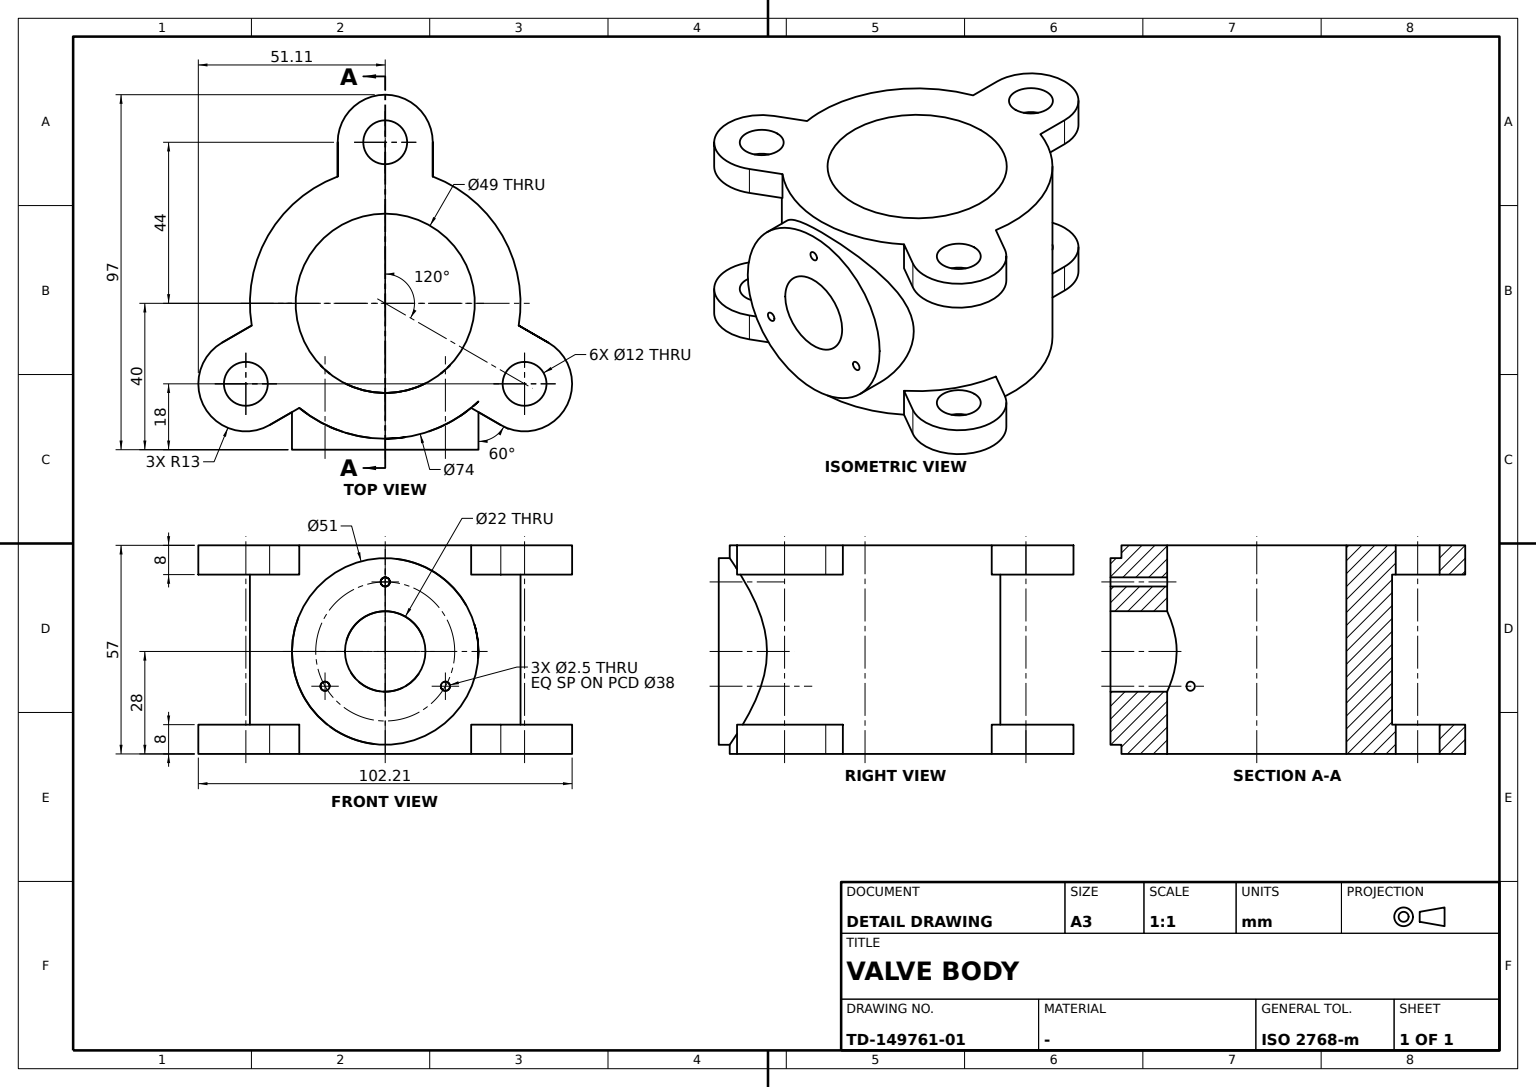
CATIA V5 part; units mm, degrees
ref_plane "Plane1" through (-40, 0, 0) normal (1, 0, 0) x (0, 1, 0)
sketch "Sketch1" plane through (0, 0, 0) normal (0, 0, 1) x (1, 0, 0)
  circle A0 centre (0, 0) radius 37
  dimension "radius A0" = 37
extrude "Pad1" add sketch "Sketch1" along normal blind 57
sketch "Sketch2" plane through (0, 0, 57) normal (0, 0, 1) x (1, 0, 0)
  circle A0 centre (0, 0) radius 24.5
  dimension "radius A0" = 24.5
extrude "Pocket1" cut sketch "Sketch2" against normal blind 57
sketch "Sketch3" plane through (0, 0, 57) normal (0, 0, 1) x (1, 0, 0)
  circle A0 centre (44, 0) radius 6
  point P0 (44, 0)
  arc A1 (44, -13) -> (44, 13) centre (44, 0) ccw
  line L0 (34.641, 13) -> (44, 13)
  point P1 (34.641, 13)
  line L1 (34.641, -13) -> (44, -13)
  point P2 (34.641, -13)
  circle A2 centre (0, 0) radius 37 construction
  arc A3 (-6.0622, 36.5) -> (-28.5788, 23.5) centre (0, 0) ccw
  arc A4 (34.641, -13) -> (34.641, 13) centre (0, 0) ccw
  arc A5 (-28.5788, -23.5) -> (-6.0622, -36.5) centre (0, 0) ccw
  line L2 (0, 0) -> (-22, 38.1051) construction
  point P3 (-22, 38.1051)
  circle A6 centre (-22, 38.1051) radius 6
  point P4 (-22, 38.1051)
  arc A7 (-10.7417, 44.6051) -> (-33.2583, 31.6051) centre (-22, 38.1051) ccw
  line L3 (-33.2583, 31.6051) -> (-28.5788, 23.5)
  point P5 (-28.5788, 23.5)
  line L4 (-10.7417, 44.6051) -> (-6.0622, 36.5)
  point P6 (-6.0622, 36.5)
  point P7 (-22, -38.1051)
  point P8 (0, 0)
  line L5 (0, 0) -> (-22, -38.1051) construction
  circle A8 centre (-22, -38.1051) radius 6
  arc A9 (-33.2583, -31.6051) -> (-10.7417, -44.6051) centre (-22, -38.1051) ccw
  line L6 (-10.7417, -44.6051) -> (-6.0622, -36.5)
  point P9 (-6.0622, -36.5)
  line L7 (-33.2583, -31.6051) -> (-28.5788, -23.5)
  point P10 (-28.5788, -23.5)
  dimension "radius A0" = 6
  dimension "distance P0 y axis" = 44
  dimension "radius A1" = 13
  dimension "angle L2 x axis" = 120
  dimension "radius A6" = 6
  dimension "distance P4 origin" = 44
  dimension "radius A7" = 13
  dimension "length L5" = 44
  dimension "radius A8" = 6
  dimension "radius A9" = 13
  constraint coincidence P0 x-axis
  constraint coincidence P1 A2
  constraint coincidence P2 A2
  constraint coincidence P4 L2
  constraint coincidence P5 A2
  constraint coincidence P6 A2
  constraint coincidence P9 A2
  constraint coincidence P10 A2
  constraint horizontal L0 x-axis
  constraint horizontal L1 x-axis
  constraint tangency L0 A1
  constraint tangency L1 A1
  constraint tangency L3 A7
  constraint tangency L4 A7
  constraint tangency L6 A9
  constraint tangency L7 A9
  constraint parallelism L3 L2
  constraint parallelism L4 L2
  constraint parallelism L6 L5
  constraint parallelism L7 L5
  constraint symmetry P3 P7 x-axis
  constraint symmetry origin P8 x-axis
  constraint symmetry L2 L5 x-axis
  constraint concentricity A9 A8
extrude "Pad2" add sketch "Sketch3" against normal blind 8
sketch "Sketch4" plane through (0, 0, 0) normal (0, 0, -1) x (1, 0, 0)
  circle A0 centre (44, 0) radius 6
  arc A1 (44, -13) -> (44, 13) centre (44, 0) ccw construction
  arc A2 (44, -13) -> (44, 13) centre (44, 0) ccw
  arc A3 (-10.7417, 44.6051) -> (-33.2583, 31.6051) centre (-22, 38.1051) ccw
  circle A4 centre (-22, 38.1051) radius 6
  circle A5 centre (-22, -38.1051) radius 6
  arc A6 (-33.2583, -31.6051) -> (-10.7417, -44.6051) centre (-22, -38.1051) ccw
  circle A7 centre (-22, 38.1051) radius 6 construction
  arc A8 (-10.7417, 44.6051) -> (-33.2583, 31.6051) centre (-22, 38.1051) ccw construction
  circle A9 centre (-22, -38.1051) radius 6 construction
  arc A10 (-33.2583, -31.6051) -> (-10.7417, -44.6051) centre (-22, -38.1051) ccw construction
  line L0 (-33.2583, 31.6051) -> (-28.5788, 23.5)
  point P0 (-28.5788, 23.5)
  line L1 (-28.5788, 23.5) -> (-33.2583, 31.6051) construction
  circle A11 centre (0, 0) radius 37 construction
  arc A12 (34.641, -13) -> (34.641, 13) centre (0, 0) ccw
  arc A13 (-6.0622, 36.5) -> (-28.5788, 23.5) centre (0, 0) ccw
  arc A14 (-28.5788, -23.5) -> (-6.0622, -36.5) centre (0, 0) ccw
  line L2 (-10.7417, 44.6051) -> (-6.0622, 36.5)
  point P1 (-6.0622, 36.5)
  line L3 (-10.7417, 44.6051) -> (-6.0622, 36.5) construction
  line L4 (34.641, 13) -> (44, 13)
  point P2 (34.641, 13)
  line L5 (34.641, -13) -> (44, -13)
  point P3 (34.641, -13)
  line L6 (-10.7417, -44.6051) -> (-6.0622, -36.5)
  point P4 (-6.0622, -36.5)
  line L7 (-6.0622, -36.5) -> (-10.7417, -44.6051) construction
  line L8 (-33.2583, -31.6051) -> (-28.5788, -23.5)
  point P5 (-28.5788, -23.5)
  line L9 (-33.2583, -31.6051) -> (-28.5788, -23.5) construction
  dimension "radius A0" = 6
  dimension "radius A6" = 13
  dimension "radius A5" = 6
  dimension "radius A2" = 13
  dimension "radius A4" = 6
  dimension "radius A3" = 13
  constraint concentricity A0 A1
  constraint concentricity A2 A1
  constraint concentricity A4 A7
  constraint concentricity A3 A8
  constraint concentricity A5 A9
  constraint concentricity A6 A10
  constraint parallelism L0 L1
  constraint parallelism L3 L2
  constraint parallelism L6 L7
  constraint parallelism L8 L9
  constraint tangency L0 A3
  constraint tangency L2 A3
  constraint tangency L4 A2
  constraint tangency L5 A2
  constraint tangency L6 A6
  constraint tangency L8 A6
  constraint coincidence P0 A11
  constraint coincidence P1 A11
  constraint coincidence P2 A11
  constraint coincidence P3 A11
  constraint coincidence P4 A11
  constraint coincidence P5 A11
  constraint horizontal L4 x-axis
  constraint horizontal L5 x-axis
extrude "Pad3" add sketch "Sketch4" against normal blind 8
sketch "Sketch5" plane through (-40, 0, 0) normal (1, 0, 0) x (0, 1, 0)
  circle A0 centre (0, 28) radius 25.5
  point P0 (0, 28)
  line L0 (37, 57) -> (-37, 57) construction
  dimension "radius A0" = 25.5
  dimension "distance P0 L0" = 29
  constraint coincidence P0 y-axis
extrude "Pad4" add sketch "Sketch5" along normal up to surface face at (20.4755, 30.8181, 46.93)
sketch "Sketch6" plane through (-40, 0, 0) normal (-1, 0, 0) x (0, -1, 0)
  circle A0 centre (0, 28) radius 11
  circle A1 centre (0, 28) radius 25.5 construction
  dimension "radius A0" = 11
  constraint concentricity A0 A1
extrude "Pocket2" cut sketch "Sketch6" against normal up to surface (40 mm away)
sketch "Sketch7" plane through (-40, 0, 0) normal (-1, 0, 0) x (0, -1, 0)
  circle A0 centre (0, 28) radius 19 construction
  circle A1 centre (0, 28) radius 25.5 construction
  circle A2 centre (0, 47) radius 1.25
  point P0 (0, 47)
  line L0 (0, 28) -> (-58.3905, -5.7118) construction
  circle A3 centre (-16.4545, 18.5) radius 1.25
  point P1 (-16.4545, 18.5)
  circle A4 centre (16.4545, 18.5) radius 1.25
  dimension "radius A0" = 19
  dimension "radius A2" = 1.25
  dimension "angle y axis L0" = 120
  dimension "radius A3" = 1.25
  constraint concentricity A0 A1
  constraint coincidence P0 A0
  constraint coincidence P0 y-axis
  constraint coincidence P1 L0
  constraint coincidence P1 A0
  constraint symmetry A3 A4 y-axis
extrude "Pocket3" cut sketch "Sketch7" against normal up to surface (40 mm away)
